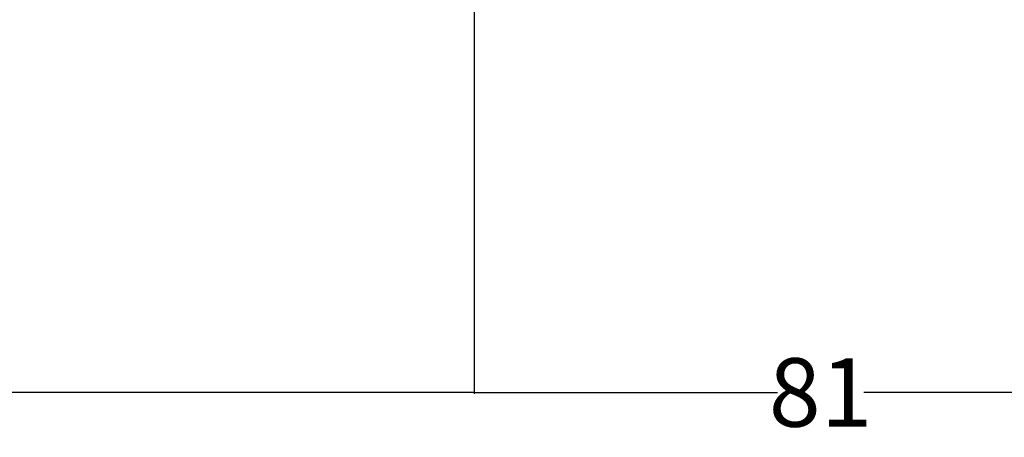
# Model space of a CAD drawing. Units: inches. Extents: x -48 to 50072, y 0 to 21068.
# Tile 3 of 75: x 163 to 278, y 161 to 210. Entities that reach past the tile are written whole.
import ezdxf

# ---------------------------------------------------------------- set-up
doc = ezdxf.new("R2010")
doc.units = ezdxf.units.IN
doc.header["$MEASUREMENT"] = 0
doc.layers.add('A-ANNO-DIMS', color=2, linetype='Continuous', lineweight=18)
doc.styles.get("Standard").update_dxf_attribs({"font": 'arial.ttf'})
doc.dimstyles.get("Standard").update_dxf_attribs({"dimtxt": 8, "dimasz": 0.18, "dimexe": 0.18, "dimexo": 0.0625, "dimgap": 0.09, "dimtad": 0, "dimtih": 1, "dimtoh": 1, "dimdec": 1, "dimzin": 0, "dimdsep": 46, "dimlunit": 4, "dimtxsty": 'Standard', "dimblk": 'ARCHTICK', "dimcen": 0.09, "dimadec": 0, "dimazin": 0, "dimtfac": 1, "dimtdec": 1, "dimtofl": 0, "dimtmove": 0, "dimatfit": 3, "dimldrblk": 'ARCHTICK', "dimfxl": 1, "dimtolj": 1, "dimtzin": 0, "dimarcsym": 0})

# ---------------------------------------------------------------- blocks, each defined once
blk = doc.blocks.new('_ArchTick')
at = {"color": 0, "linetype": 'ByBlock', "const_width": 0.15}
blk.add_lwpolyline([(-0.5, -0.5), (0.5, 0.5)], dxfattribs=at)
blk = doc.blocks.new('*D116')
at = {"layer": 'A-ANNO-DIMS', "color": 0, "lineweight": -2, "transparency": 16777216}
for p, q in [((18.02, 677.71), (18.02, 165.94)), ((216.02, 677.71), (216.02, 165.94)), ((18.02, 166.12), (108.46, 166.12)), ((216.02, 166.12), (125.58, 166.12))]:
    blk.add_line(p, q, dxfattribs=at)
at = {"layer": 'Defpoints', "color": 0, "transparency": 16777216}
for p in [(18.02, 677.77), (216.02, 677.77), (216.02, 166.12)]:
    blk.add_point(p, dxfattribs=at)
at = {"layer": 'A-ANNO-DIMS', "color": 0, "lineweight": -2, "transparency": 16777216, "xscale": 0.18, "yscale": 0.18, "zscale": 0.18, "rotation": 180}
blk.add_blockref('_ArchTick', (18.02, 166.12), dxfattribs=at)
at = {"layer": 'A-ANNO-DIMS', "color": 0, "lineweight": -2, "transparency": 16777216, "xscale": 0.18, "yscale": 0.18, "zscale": 0.18}
blk.add_blockref('_ArchTick', (216.02, 166.12), dxfattribs=at)
at = {"layer": 'A-ANNO-DIMS', "color": 0, "transparency": 16777216, "insert": (117.02, 166.12), "char_height": 8, "attachment_point": 5}
blk.add_mtext('\\A1;198', dxfattribs=at)
blk = doc.blocks.new('*D117')
at = {"layer": 'A-ANNO-DIMS', "color": 0, "lineweight": -2, "transparency": 16777216}
for p, q in [((216.02, 488.71), (216.02, 165.94)), ((297.02, 488.71), (297.02, 165.94)), ((216.02, 166.12), (251.46, 166.12)), ((297.02, 166.12), (261.57, 166.12))]:
    blk.add_line(p, q, dxfattribs=at)
at = {"layer": 'Defpoints', "color": 0, "transparency": 16777216}
for p in [(216.02, 488.77), (297.02, 488.77), (297.02, 166.12)]:
    blk.add_point(p, dxfattribs=at)
at = {"layer": 'A-ANNO-DIMS', "color": 0, "lineweight": -2, "transparency": 16777216, "xscale": 0.18, "yscale": 0.18, "zscale": 0.18, "rotation": 180}
blk.add_blockref('_ArchTick', (216.02, 166.12), dxfattribs=at)
at = {"layer": 'A-ANNO-DIMS', "color": 0, "lineweight": -2, "transparency": 16777216, "xscale": 0.18, "yscale": 0.18, "zscale": 0.18}
blk.add_blockref('_ArchTick', (297.02, 166.12), dxfattribs=at)
at = {"layer": 'A-ANNO-DIMS', "color": 0, "transparency": 16777216, "insert": (256.52, 166.12), "char_height": 8, "attachment_point": 5}
blk.add_mtext('\\A1;81', dxfattribs=at)

msp = doc.modelspace()

# ---------------------------------------------------------------- dimensions: what is measured, and where the dimension line sits
at = {"layer": 'A-ANNO-DIMS'}
for base, p1, p2, picture, middle in [((216.017, 166.125), (18.017, 677.775), (216.017, 677.775), '*D116', (117.017, 166.125)), ((297.017, 166.125), (216.017, 488.775), (297.017, 488.775), '*D117', (256.517, 166.125))]:
    dim = msp.add_linear_dim(base=base, p1=p1, p2=p2, dimstyle='Standard', override={"dimdec": 0, "dimlfac": 1, "dimrnd": 0, "dimzin": 0, "dimdsep": 46, "dimlunit": 2}, dxfattribs=at)
    dim.commit()
    dim.dimension.update_dxf_attribs({"geometry": picture, "text_midpoint": middle})

doc.saveas('drawing.dxf')
